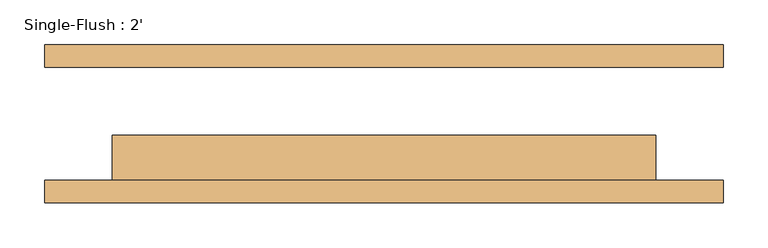
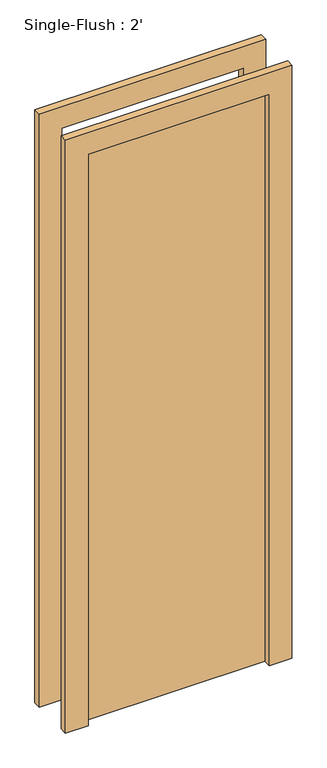
"""IFC4 building model written with IfcOpenShell, lengths in millimetres: door geometry, Single-Flush : 2'."""

from ifc_helpers import new_model, si_unit, frame, origin, origin_with_axes, place, context, project, spatial, polyline, outline, extrude, source, transform, mapped, element, save


def single_flush_2_ccebbf4d(model_context):
    return source(origin(), model_context, "Body", "SweptSolid", [
        extrude(outline(polyline([(2108.2, -381.0), (0.0, -381.0), (0.0, -304.8), (2032.0, -304.8), (2032.0, 304.8), (0.0, 304.8), (0.0, 381.0), (2108.2, 381.0), (2108.2, -381.0)])), frame((0.0, -88.9, 0.0), z_axis=(0.0, 1.0, 0.0), x_axis=(0.0, 0.0, 1.0)), (0.0, 0.0, 1.0), 25.4),
        extrude(outline(polyline([(2108.2, 381.0), (2108.2, -381.0), (0.0, -381.0), (0.0, -304.8), (2032.0, -304.8), (2032.0, 304.8), (0.0, 304.8), (0.0, 381.0), (2108.2, 381.0)])), frame((0.0, 63.5, 0.0), z_axis=(0.0, 1.0, 0.0), x_axis=(0.0, 0.0, 1.0)), (0.0, 0.0, 1.0), 25.4),
        extrude(outline(polyline([(304.8, -12.7), (304.8, -63.5), (-304.8, -63.5), (-304.8, -12.7), (304.8, -12.7)])), origin_with_axes(), (0.0, 0.0, 1.0), 2032.0),
    ])


if __name__ == "__main__":
    model = new_model("IFC4")
    model_context = context("Model", 3, world=origin())
    ifc_project = project(units=[si_unit("LENGTHUNIT", "METRE", prefix="MILLI")], contexts=[model_context])
    site = spatial("IfcSite", under=ifc_project)
    building = spatial("IfcBuilding", under=site)
    placement = place(None, origin())
    single_flush_2_shape = single_flush_2_ccebbf4d(model_context)
    element("IfcDoor", 1, ObjectType="Single-Flush : 2'", at=placement, inside=building, context=model_context, shape_type="MappedRepresentation", body=[
        mapped(single_flush_2_shape, transform((0.0, 0.0, 0.0), x_axis=(1.0, 0.0, 0.0), y_axis=(0.0, 1.0, 0.0), z_axis=(0.0, 0.0, 1.0))),
    ])
    save(model, "model.ifc")

# Revit data of these elements
# Type "Single-Flush : 2'"
#   Type Mark = "8"
#   Construction Type Id = "MDOOR"
#   Assembly Code = "C1020"
#   Analytic Construction = "Metal"
#   Thickness = 0' - 2"
#   Heat Transfer Coefficient (U) = 0.651978 BTU/(h·ft²·°F)
#   Height = 6' - 8"
#   Trim Projection Ext = 0' - 1"
#   Trim Projection Int = 0' - 1"
#   Trim Width = 0' - 3"
#   Width = 2' - 0"
#   Define Thermal Properties by = 1
#   Door Material = Door - Panel
#   Frame Material = Door - Frame
#   Visual Light Transmittance = 0
#   Solar Heat Gain Coefficient = 0
#   Function = (empty or 0)
#   Wall Closure = (empty or 0)
# Element 1 (IfcDoor, "Single-Flush : 2'")
#   Materials on its faces: "Door - Frame", "Door - Panel"
# Materials
#   "Door - Panel": class "Wood", colour RGB 210 159 95, transparency 0, Cost = 0
#   "Door - Frame": colour RGB 118 70 51, transparency 0, Cost = 0
